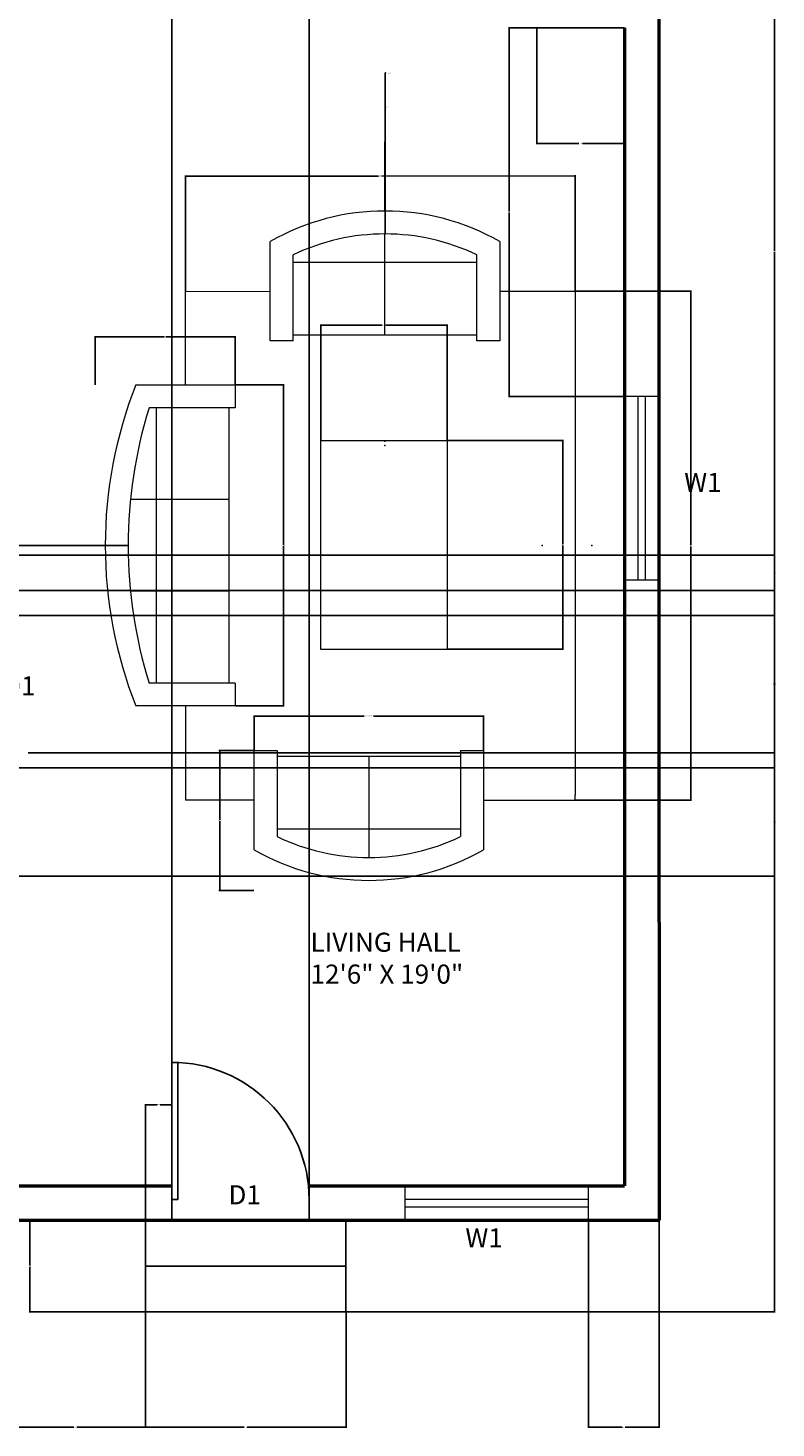
# Model space of a CAD drawing. Units: inches. Extents: x 437 to 811, y 2074 to 2699.
# Tile 2 of 4: x 615 to 811, y 2074 to 2441. Entities that reach past the tile are written whole.
import ezdxf

# ---------------------------------------------------------------- set-up
doc = ezdxf.new("R2010")
doc.units = ezdxf.units.IN
for name, color, linetype, lineweight in [('A-ANNO-DIMS', 2, 'Continuous', 18), ('A-ANNO-TEXT', 7, 'Continuous', 18), ('A-AREA-IDEN', 7, 'Continuous', 25), ('A-DOOR', 4, 'Continuous', 25), ('A-FLOR-STRS', 7, 'Continuous', 25), ('A-FURN', 8, 'Continuous', 18), ('A-GLAZ', 4, 'Continuous', 18), ('A-WALL', 7, 'Continuous', 50)]:
    doc.layers.add(name, color=color, linetype=linetype, lineweight=lineweight)
doc.styles.get("Standard").update_dxf_attribs({"font": 'arial.ttf'})
doc.dimstyles.get("Standard").update_dxf_attribs({"dimtxt": 0.18, "dimasz": 0.18, "dimexe": 0.18, "dimexo": 0.0625, "dimgap": 0.09, "dimtad": 0, "dimtih": 1, "dimtoh": 1, "dimdec": 4, "dimzin": 0, "dimdsep": 46, "dimtxsty": 'Standard', "dimcen": 0.09, "dimadec": 0, "dimazin": 0, "dimtfac": 1, "dimtdec": 4, "dimtofl": 0, "dimtmove": 0, "dimatfit": 3, "dimfxl": 1, "dimtolj": 1, "dimtzin": 0, "dimarcsym": 0})

# ---------------------------------------------------------------- blocks, each defined once
blk = doc.blocks.new('Sofa - Roundback 7 ft.')
for p, q in [((-12.00002, -32.4421), (-12.00003, -6.5971)), ((11.99997, -32.4421), (11.99998, -6.5971)), ((-36.000027, -34), (-36.000027, -11.4696)), ((-35.999844, -13.3819), (35.9998, -13.3819)), ((35.99998, -34), (35.99998, -11.4696)), ((-36.000027, -32.4421), (35.99998, -32.4421))]:
    blk.add_line(p, q)
for points in [[(-36.000027, -34), (-42.000027, -34), (-42.000027, -8)], [(41.99998, -8), (41.99998, -34), (35.99998, -34)]]:
    blk.add_lwpolyline(points)
for centre, radius, start, end in [((0, -114.25), 114.25, 68.43141, 111.5686), ((-0.00001, -127.1968), 121.1968, 72.72033, 107.2797)]:
    blk.add_arc(centre, radius, start, end)
blk = doc.blocks.new('Sofa - Roundback Loveseat 5 ft.')
for p, q in [((0, -32.44198), (0, -5.99998)), ((-24, -33.99998), (-24, -11.46958)), ((-23.9998, -13.38178), (23.99986, -13.38178)), ((24.00004, -33.99998), (24.00004, -11.46958)), ((-24, -32.44198), (24.00004, -32.44198))]:
    blk.add_line(p, q)
for points in [[(-24, -33.99998), (-30, -33.99998), (-30, -7.99998)], [(30.00004, -7.99998), (30.00004, -33.99998), (24.00004, -33.99998)]]:
    blk.add_lwpolyline(points)
for centre, radius, start, end in [((0, -60.24998), 60.24998, 60.13715, 119.8628), ((0, -61.38438), 55.38444, 64.32083, 115.6792)]:
    blk.add_arc(centre, radius, start, end)
blk = doc.blocks.new('*U10')
for p, q in [((0, 0), (0, -6)), ((40, 0), (40, -6))]:
    blk.add_line(p, q)
blk.add_lwpolyline([(0, 0), (0, 40), (1.75, 40), (1.75, 0)], close=True)
blk.add_arc((0, 0), 40, 0, 90)
blk = doc.blocks.new('WIN-W1-48IN')
for p, q in [((0, 5.5), (48, 5.5)), ((0, 3.5), (48, 3.5))]:
    blk.add_line(p, q)
blk.add_lwpolyline([(0, 0), (48, 0), (48, 9), (0, 9)], close=True)
blk = doc.blocks.new('*D26')
at = {"layer": 'A-ANNO-DIMS', "color": 0, "lineweight": -2, "transparency": 16777216}
for p, q in [((674.12, 2251.79), (674.12, 2260.91)), ((674.3, 2260.73), (702.89, 2260.73)), ((733.94, 2260.73), (705.34, 2260.73)), ((734.12, 2251.79), (734.12, 2260.91))]:
    blk.add_line(p, q, dxfattribs=at)
at = {"layer": 'A-ANNO-DIMS', "color": 0, "transparency": 16777216}
for points in [[(674.3, 2260.76), (674.3, 2260.7), (674.12, 2260.73)], [(733.94, 2260.76), (733.94, 2260.7), (734.12, 2260.73)]]:
    blk.add_solid(points, dxfattribs=at)
at = {"layer": 'Defpoints', "color": 0, "transparency": 16777216}
for p in [(674.12, 2260.73), (674.12, 2251.73), (734.12, 2251.73)]:
    blk.add_point(p, dxfattribs=at)
at = {"layer": 'A-ANNO-DIMS', "color": 0, "transparency": 16777216, "insert": (704.12, 2260.73), "char_height": 0.18, "attachment_point": 5}
blk.add_mtext('\\A1;LOVESEAT 60 TYP.', dxfattribs=at)
blk = doc.blocks.new('*D27')
at = {"layer": 'A-ANNO-DIMS', "color": 0, "lineweight": -2, "transparency": 16777216}
for p, q in [((674.05, 2251.73), (664.94, 2251.73)), ((665.12, 2251.55), (665.12, 2233.58)), ((665.12, 2215.25), (665.12, 2233.22)), ((674.05, 2215.07), (664.94, 2215.07))]:
    blk.add_line(p, q, dxfattribs=at)
at = {"layer": 'A-ANNO-DIMS', "color": 0, "transparency": 16777216}
for points in [[(665.09, 2251.55), (665.15, 2251.55), (665.12, 2251.73)], [(665.09, 2215.25), (665.15, 2215.25), (665.12, 2215.07)]]:
    blk.add_solid(points, dxfattribs=at)
at = {"layer": 'Defpoints', "color": 0, "transparency": 16777216}
for p in [(674.12, 2251.73), (665.12, 2215.07), (674.12, 2215.07)]:
    blk.add_point(p, dxfattribs=at)
at = {"layer": 'A-ANNO-DIMS', "color": 0, "transparency": 16777216, "insert": (665.12, 2233.4), "char_height": 0.18, "attachment_point": 5}
blk.add_mtext('\\A1;37 TYP.', dxfattribs=at)
blk = doc.blocks.new('*D36')
at = {"layer": 'A-ANNO-DIMS', "color": 0, "lineweight": -2, "transparency": 16777216}
for p, q in [((669.25, 2347.38), (681.97, 2347.38)), ((681.79, 2347.2), (681.79, 2305.57)), ((681.79, 2263.56), (681.79, 2305.2)), ((669.25, 2263.38), (681.97, 2263.38))]:
    blk.add_line(p, q, dxfattribs=at)
at = {"layer": 'A-ANNO-DIMS', "color": 0, "transparency": 16777216}
for points in [[(681.76, 2347.2), (681.82, 2347.2), (681.79, 2347.38)], [(681.76, 2263.56), (681.82, 2263.56), (681.79, 2263.38)]]:
    blk.add_solid(points, dxfattribs=at)
at = {"layer": 'Defpoints', "color": 0, "transparency": 16777216}
for p in [(669.19, 2347.38), (681.79, 2347.38), (669.19, 2263.38)]:
    blk.add_point(p, dxfattribs=at)
at = {"layer": 'A-ANNO-DIMS', "color": 0, "transparency": 16777216, "insert": (681.79, 2305.38), "char_height": 0.18, "attachment_point": 5}
blk.add_mtext('\\A1;SOFA 84', dxfattribs=at)
blk = doc.blocks.new('*D37')
at = {"layer": 'A-ANNO-DIMS', "color": 0, "lineweight": -2, "transparency": 16777216}
for p, q in [((632.53, 2347.44), (632.53, 2360.16)), ((632.71, 2359.98), (650.64, 2359.98)), ((669.01, 2359.98), (651.08, 2359.98)), ((669.19, 2347.44), (669.19, 2360.16))]:
    blk.add_line(p, q, dxfattribs=at)
at = {"layer": 'A-ANNO-DIMS', "color": 0, "transparency": 16777216}
for points in [[(632.71, 2360.01), (632.71, 2359.95), (632.53, 2359.98)], [(669.01, 2360.01), (669.01, 2359.95), (669.19, 2359.98)]]:
    blk.add_solid(points, dxfattribs=at)
at = {"layer": 'Defpoints', "color": 0, "transparency": 16777216}
for p in [(632.53, 2359.98), (632.53, 2347.38), (669.19, 2347.38)]:
    blk.add_point(p, dxfattribs=at)
at = {"layer": 'A-ANNO-DIMS', "color": 0, "transparency": 16777216, "insert": (650.86, 2359.98), "char_height": 0.18, "attachment_point": 5}
blk.add_mtext('\\A1;37', dxfattribs=at)
blk = doc.blocks.new('*D42')
at = {"layer": 'A-ANNO-DIMS', "color": 0, "lineweight": -2, "transparency": 16777216}
for p, q in [((645.63, 2128.8), (615.31, 2128.8)), ((615.49, 2128.62), (615.49, 2116.98)), ((615.49, 2104.98), (615.49, 2116.62)), ((645.63, 2104.8), (615.31, 2104.8))]:
    blk.add_line(p, q, dxfattribs=at)
at = {"layer": 'A-ANNO-DIMS', "color": 0, "transparency": 16777216}
for points in [[(615.46, 2128.62), (615.52, 2128.62), (615.49, 2128.8)], [(615.46, 2104.98), (615.52, 2104.98), (615.49, 2104.8)]]:
    blk.add_solid(points, dxfattribs=at)
at = {"layer": 'Defpoints', "color": 0, "transparency": 16777216}
for p in [(615.49, 2128.8), (645.69, 2128.8), (645.69, 2104.8)]:
    blk.add_point(p, dxfattribs=at)
at = {"layer": 'A-ANNO-DIMS', "color": 0, "transparency": 16777216, "insert": (615.49, 2116.8), "char_height": 0.18, "attachment_point": 5}
blk.add_mtext('\\A1;24', dxfattribs=at)
blk = doc.blocks.new('*D43')
at = {"layer": 'A-ANNO-DIMS', "color": 0, "lineweight": -2, "transparency": 16777216}
for p, q in [((645.69, 2104.74), (645.69, 2074.42)), ((698.15, 2104.74), (698.15, 2074.42)), ((645.87, 2074.6), (671.53, 2074.6)), ((697.97, 2074.6), (672.31, 2074.6))]:
    blk.add_line(p, q, dxfattribs=at)
at = {"layer": 'A-ANNO-DIMS', "color": 0, "transparency": 16777216}
for points in [[(645.87, 2074.63), (645.87, 2074.57), (645.69, 2074.6)], [(697.97, 2074.63), (697.97, 2074.57), (698.15, 2074.6)]]:
    blk.add_solid(points, dxfattribs=at)
at = {"layer": 'Defpoints', "color": 0, "transparency": 16777216}
for p in [(645.69, 2104.8), (698.15, 2104.8), (698.15, 2074.6)]:
    blk.add_point(p, dxfattribs=at)
at = {"layer": 'A-ANNO-DIMS', "color": 0, "transparency": 16777216, "insert": (671.92, 2074.6), "char_height": 0.18, "attachment_point": 5}
blk.add_mtext('\\A1;52.46', dxfattribs=at)
blk = doc.blocks.new('*D44')
at = {"layer": 'A-ANNO-DIMS', "color": 0, "lineweight": -2, "transparency": 16777216}
for p, q in [((609, 2137.74), (609, 2074.42)), ((645.69, 2104.74), (645.69, 2074.42)), ((609.18, 2074.6), (626.95, 2074.6)), ((645.51, 2074.6), (627.74, 2074.6))]:
    blk.add_line(p, q, dxfattribs=at)
at = {"layer": 'A-ANNO-DIMS', "color": 0, "transparency": 16777216}
for points in [[(609.18, 2074.63), (609.18, 2074.57), (609, 2074.6)], [(645.51, 2074.63), (645.51, 2074.57), (645.69, 2074.6)]]:
    blk.add_solid(points, dxfattribs=at)
at = {"layer": 'Defpoints', "color": 0, "transparency": 16777216}
for p in [(609, 2137.8), (645.69, 2104.8), (645.69, 2074.6)]:
    blk.add_point(p, dxfattribs=at)
at = {"layer": 'A-ANNO-DIMS', "color": 0, "transparency": 16777216, "insert": (627.35, 2074.6), "char_height": 0.18, "attachment_point": 5}
blk.add_mtext('\\A1;36.69', dxfattribs=at)
blk = doc.blocks.new('*D45')
at = {"layer": 'A-ANNO-DIMS', "color": 0, "lineweight": -2, "transparency": 16777216}
for p, q in [((652.6, 2128.86), (652.6, 2690.18)), ((652.78, 2690), (670.09, 2690)), ((688.34, 2690), (671.02, 2690)), ((688.52, 2128.86), (688.52, 2690.18))]:
    blk.add_line(p, q, dxfattribs=at)
at = {"layer": 'A-ANNO-DIMS', "color": 0, "transparency": 16777216}
for points in [[(652.78, 2690.03), (652.78, 2689.97), (652.6, 2690)], [(688.34, 2690.03), (688.34, 2689.97), (688.52, 2690)]]:
    blk.add_solid(points, dxfattribs=at)
at = {"layer": 'Defpoints', "color": 0, "transparency": 16777216}
for p in [(688.52, 2690), (652.6, 2128.8), (688.52, 2128.8)]:
    blk.add_point(p, dxfattribs=at)
at = {"layer": 'A-ANNO-DIMS', "color": 0, "transparency": 16777216, "insert": (670.56, 2690), "char_height": 0.18, "attachment_point": 5}
blk.add_mtext('\\A1;35.924', dxfattribs=at)
blk = doc.blocks.new('*D46')
at = {"layer": 'A-ANNO-DIMS', "color": 0, "lineweight": -2, "transparency": 16777216}
for p, q in [((645.69, 2128.86), (645.69, 2159.18)), ((645.87, 2159), (648.75, 2159)), ((652.42, 2159), (649.54, 2159)), ((652.6, 2128.86), (652.6, 2159.18))]:
    blk.add_line(p, q, dxfattribs=at)
at = {"layer": 'A-ANNO-DIMS', "color": 0, "transparency": 16777216}
for points in [[(645.87, 2159.03), (645.87, 2158.97), (645.69, 2159)], [(652.42, 2159.03), (652.42, 2158.97), (652.6, 2159)]]:
    blk.add_solid(points, dxfattribs=at)
at = {"layer": 'Defpoints', "color": 0, "transparency": 16777216}
for p in [(652.6, 2159), (645.69, 2128.8), (652.6, 2128.8)]:
    blk.add_point(p, dxfattribs=at)
at = {"layer": 'A-ANNO-DIMS', "color": 0, "transparency": 16777216, "insert": (649.14, 2159), "char_height": 0.18, "attachment_point": 5}
blk.add_mtext('\\A1;6.903', dxfattribs=at)
blk = doc.blocks.new('*D47')
at = {"layer": 'A-ANNO-DIMS', "color": 0, "lineweight": -2, "transparency": 16777216}
for p, q in [((761.56, 2128.74), (761.56, 2074.42)), ((780, 2128.74), (780, 2074.42)), ((761.74, 2074.6), (770.4, 2074.6)), ((779.82, 2074.6), (771.17, 2074.6))]:
    blk.add_line(p, q, dxfattribs=at)
at = {"layer": 'A-ANNO-DIMS', "color": 0, "transparency": 16777216}
for points in [[(761.74, 2074.63), (761.74, 2074.57), (761.56, 2074.6)], [(779.82, 2074.63), (779.82, 2074.57), (780, 2074.6)]]:
    blk.add_solid(points, dxfattribs=at)
at = {"layer": 'Defpoints', "color": 0, "transparency": 16777216}
for p in [(761.56, 2128.8), (780, 2128.8), (780, 2074.6)]:
    blk.add_point(p, dxfattribs=at)
at = {"layer": 'A-ANNO-DIMS', "color": 0, "transparency": 16777216, "insert": (770.78, 2074.6), "char_height": 0.18, "attachment_point": 5}
blk.add_mtext('\\A1;18.44', dxfattribs=at)
blk = doc.blocks.new('*D55')
at = {"layer": 'A-ANNO-DIMS', "color": 0, "lineweight": -2, "transparency": 16777216}
for p, q in [((770.94, 2440.8), (740.62, 2440.8)), ((740.8, 2440.62), (740.8, 2392.78)), ((740.8, 2344.57), (740.8, 2392.41)), ((770.94, 2344.39), (740.62, 2344.39))]:
    blk.add_line(p, q, dxfattribs=at)
at = {"layer": 'A-ANNO-DIMS', "color": 0, "transparency": 16777216}
for points in [[(740.77, 2440.62), (740.83, 2440.62), (740.8, 2440.8)], [(740.77, 2344.57), (740.83, 2344.57), (740.8, 2344.39)]]:
    blk.add_solid(points, dxfattribs=at)
at = {"layer": 'Defpoints', "color": 0, "transparency": 16777216}
for p in [(740.8, 2440.8), (771, 2440.8), (771, 2344.39)]:
    blk.add_point(p, dxfattribs=at)
at = {"layer": 'A-ANNO-DIMS', "color": 0, "transparency": 16777216, "insert": (740.8, 2392.59), "char_height": 0.18, "attachment_point": 5}
blk.add_mtext('\\A1;96.4', dxfattribs=at)
blk = doc.blocks.new('*D64')
at = {"layer": 'A-ANNO-DIMS', "color": 0, "lineweight": -2, "transparency": 16777216}
for p, q in [((615.07, 2287.06), (810.38, 2287.06)), ((810.2, 2286.88), (810.2, 2269.28)), ((810.2, 2251.31), (810.2, 2268.91)), ((615.07, 2251.13), (810.38, 2251.13))]:
    blk.add_line(p, q, dxfattribs=at)
at = {"layer": 'A-ANNO-DIMS', "color": 0, "transparency": 16777216}
for points in [[(810.17, 2286.88), (810.23, 2286.88), (810.2, 2287.06)], [(810.17, 2251.31), (810.23, 2251.31), (810.2, 2251.13)]]:
    blk.add_solid(points, dxfattribs=at)
at = {"layer": 'Defpoints', "color": 0, "transparency": 16777216}
for p in [(615, 2287.06), (810.2, 2287.06), (615, 2251.13)]:
    blk.add_point(p, dxfattribs=at)
at = {"layer": 'A-ANNO-DIMS', "color": 0, "transparency": 16777216, "insert": (810.2, 2269.1), "char_height": 0.18, "attachment_point": 5}
blk.add_mtext('\\A1;35.924', dxfattribs=at)
blk = doc.blocks.new('*D65')
at = {"layer": 'A-ANNO-DIMS', "color": 0, "lineweight": -2, "transparency": 16777216}
for p, q in [((609.07, 2302.8), (810.38, 2302.8)), ((810.2, 2302.62), (810.2, 2295.11)), ((810.2, 2287.23), (810.2, 2294.74)), ((609.07, 2287.05), (810.38, 2287.05))]:
    blk.add_line(p, q, dxfattribs=at)
at = {"layer": 'A-ANNO-DIMS', "color": 0, "transparency": 16777216}
for points in [[(810.17, 2302.62), (810.23, 2302.62), (810.2, 2302.8)], [(810.17, 2287.23), (810.23, 2287.23), (810.2, 2287.05)]]:
    blk.add_solid(points, dxfattribs=at)
at = {"layer": 'Defpoints', "color": 0, "transparency": 16777216}
for p in [(609, 2302.8), (810.2, 2302.8), (609, 2287.05)]:
    blk.add_point(p, dxfattribs=at)
at = {"layer": 'A-ANNO-DIMS', "color": 0, "transparency": 16777216, "insert": (810.2, 2294.93), "char_height": 0.18, "attachment_point": 5}
blk.add_mtext('\\A1;15.747', dxfattribs=at)
blk = doc.blocks.new('*D68')
at = {"layer": 'A-ANNO-DIMS', "color": 0, "lineweight": -2, "transparency": 16777216}
for p, q in [((609.07, 2247.18), (810.38, 2247.18)), ((810.2, 2247), (810.2, 2233.17)), ((810.2, 2218.98), (810.2, 2232.81)), ((609.07, 2218.8), (810.38, 2218.8))]:
    blk.add_line(p, q, dxfattribs=at)
at = {"layer": 'A-ANNO-DIMS', "color": 0, "transparency": 16777216}
for points in [[(810.17, 2247), (810.23, 2247), (810.2, 2247.18)], [(810.17, 2218.98), (810.23, 2218.98), (810.2, 2218.8)]]:
    blk.add_solid(points, dxfattribs=at)
at = {"layer": 'Defpoints', "color": 0, "transparency": 16777216}
for p in [(609, 2247.18), (810.2, 2247.18), (609, 2218.8)]:
    blk.add_point(p, dxfattribs=at)
at = {"layer": 'A-ANNO-DIMS', "color": 0, "transparency": 16777216, "insert": (810.2, 2232.99), "char_height": 0.18, "attachment_point": 5}
blk.add_mtext('\\A1;28.384', dxfattribs=at)
blk = doc.blocks.new('*D70')
at = {"layer": 'A-ANNO-DIMS', "color": 0, "lineweight": -2, "transparency": 16777216}
for p, q in [((505.98, 2302.8), (810.38, 2302.8)), ((810.2, 2302.62), (810.2, 2298.36)), ((810.2, 2293.74), (810.2, 2298)), ((500.46, 2293.56), (810.38, 2293.56))]:
    blk.add_line(p, q, dxfattribs=at)
at = {"layer": 'A-ANNO-DIMS', "color": 0, "transparency": 16777216}
for points in [[(810.17, 2302.62), (810.23, 2302.62), (810.2, 2302.8)], [(810.17, 2293.74), (810.23, 2293.74), (810.2, 2293.56)]]:
    blk.add_solid(points, dxfattribs=at)
at = {"layer": 'Defpoints', "color": 0, "transparency": 16777216}
for p in [(505.92, 2302.8), (810.2, 2302.8), (500.4, 2293.56)]:
    blk.add_point(p, dxfattribs=at)
at = {"layer": 'A-ANNO-DIMS', "color": 0, "transparency": 16777216, "insert": (810.2, 2298.18), "char_height": 0.18, "attachment_point": 5}
blk.add_mtext('\\A1;9.244', dxfattribs=at)
blk = doc.blocks.new('*D78')
at = {"layer": 'A-ANNO-DIMS', "color": 0, "lineweight": -2, "transparency": 16777216}
for p, q in [((748.06, 2440.74), (748.06, 2410.42)), ((771, 2440.74), (771, 2410.42)), ((748.24, 2410.6), (759.07, 2410.6)), ((770.82, 2410.6), (760, 2410.6))]:
    blk.add_line(p, q, dxfattribs=at)
at = {"layer": 'A-ANNO-DIMS', "color": 0, "transparency": 16777216}
for points in [[(748.24, 2410.63), (748.24, 2410.57), (748.06, 2410.6)], [(770.82, 2410.63), (770.82, 2410.57), (771, 2410.6)]]:
    blk.add_solid(points, dxfattribs=at)
at = {"layer": 'Defpoints', "color": 0, "transparency": 16777216}
for p in [(748.06, 2440.8), (771, 2440.8), (748.06, 2410.6)]:
    blk.add_point(p, dxfattribs=at)
at = {"layer": 'A-ANNO-DIMS', "color": 0, "transparency": 16777216, "insert": (759.53, 2410.6), "char_height": 0.18, "attachment_point": 5}
blk.add_mtext('\\A1;22.947', dxfattribs=at)
blk = doc.blocks.new('*D82')
at = {"layer": 'A-ANNO-DIMS', "color": 0, "lineweight": -2, "transparency": 16777216}
for p, q in [((691.53, 2332.93), (691.53, 2363.24)), ((724.63, 2332.93), (724.63, 2363.24)), ((691.71, 2363.06), (707.62, 2363.06)), ((724.45, 2363.06), (708.55, 2363.06))]:
    blk.add_line(p, q, dxfattribs=at)
at = {"layer": 'A-ANNO-DIMS', "color": 0, "transparency": 16777216}
for points in [[(691.71, 2363.09), (691.71, 2363.03), (691.53, 2363.06)], [(724.45, 2363.09), (724.45, 2363.03), (724.63, 2363.06)]]:
    blk.add_solid(points, dxfattribs=at)
at = {"layer": 'Defpoints', "color": 0, "transparency": 16777216}
for p in [(724.63, 2363.06), (691.53, 2332.86), (724.63, 2332.86)]:
    blk.add_point(p, dxfattribs=at)
at = {"layer": 'A-ANNO-DIMS', "color": 0, "transparency": 16777216, "insert": (708.08, 2363.06), "char_height": 0.18, "attachment_point": 5}
blk.add_mtext('\\A1;33.096', dxfattribs=at)
blk = doc.blocks.new('*D83')
at = {"layer": 'A-ANNO-DIMS', "color": 0, "lineweight": -2, "transparency": 16777216}
for p, q in [((724.69, 2332.86), (755.01, 2332.86)), ((754.83, 2332.68), (754.83, 2305.71)), ((754.83, 2278.38), (754.83, 2305.35)), ((724.69, 2278.2), (755.01, 2278.2))]:
    blk.add_line(p, q, dxfattribs=at)
at = {"layer": 'A-ANNO-DIMS', "color": 0, "transparency": 16777216}
for points in [[(754.8, 2332.68), (754.86, 2332.68), (754.83, 2332.86)], [(754.8, 2278.38), (754.86, 2278.38), (754.83, 2278.2)]]:
    blk.add_solid(points, dxfattribs=at)
at = {"layer": 'Defpoints', "color": 0, "transparency": 16777216}
for p in [(724.63, 2332.86), (724.63, 2278.2), (754.83, 2278.2)]:
    blk.add_point(p, dxfattribs=at)
at = {"layer": 'A-ANNO-DIMS', "color": 0, "transparency": 16777216, "insert": (754.83, 2305.53), "char_height": 0.18, "attachment_point": 5}
blk.add_mtext('\\A1;54.67', dxfattribs=at)
blk = doc.blocks.new('*D84')
at = {"layer": 'A-ANNO-DIMS', "color": 0, "lineweight": -2, "transparency": 16777216}
for p, q in [((656.19, 2371.88), (656.17, 2402.2)), ((656.35, 2402.02), (706.68, 2402.06)), ((757.9, 2402.1), (707.56, 2402.06)), ((758.1, 2371.97), (758.08, 2402.28))]:
    blk.add_line(p, q, dxfattribs=at)
at = {"layer": 'A-ANNO-DIMS', "color": 0, "transparency": 16777216}
for points in [[(656.35, 2402.05), (656.35, 2401.99), (656.17, 2402.02)], [(757.9, 2402.13), (757.9, 2402.07), (758.08, 2402.1)]]:
    blk.add_solid(points, dxfattribs=at)
at = {"layer": 'Defpoints', "color": 0, "transparency": 16777216}
for p in [(758.08, 2402.1), (656.19, 2371.82), (758.1, 2371.9)]:
    blk.add_point(p, dxfattribs=at)
at = {"layer": 'A-ANNO-DIMS', "color": 0, "transparency": 16777216, "insert": (707.12, 2402.06), "char_height": 0.18, "attachment_point": 5}
blk.add_mtext('\\A1;101.91', dxfattribs=at)
blk = doc.blocks.new('*D85')
at = {"layer": 'A-ANNO-DIMS', "color": 0, "lineweight": -2, "transparency": 16777216}
for p, q in [((758.17, 2371.9), (788.48, 2371.9)), ((788.3, 2371.72), (788.3, 2305.5)), ((788.3, 2238.91), (788.3, 2305.14)), ((758.17, 2238.73), (788.48, 2238.73))]:
    blk.add_line(p, q, dxfattribs=at)
at = {"layer": 'A-ANNO-DIMS', "color": 0, "transparency": 16777216}
for points in [[(788.27, 2371.72), (788.33, 2371.72), (788.3, 2371.9)], [(788.27, 2238.91), (788.33, 2238.91), (788.3, 2238.73)]]:
    blk.add_solid(points, dxfattribs=at)
at = {"layer": 'Defpoints', "color": 0, "transparency": 16777216}
for p in [(758.1, 2371.9), (758.1, 2238.73), (788.3, 2238.73)]:
    blk.add_point(p, dxfattribs=at)
at = {"layer": 'A-ANNO-DIMS', "color": 0, "transparency": 16777216, "insert": (788.3, 2305.32), "char_height": 0.18, "attachment_point": 5}
blk.add_mtext('\\A1;133.17', dxfattribs=at)
blk = doc.blocks.new('*D87')
at = {"layer": 'A-ANNO-DIMS', "color": 0, "lineweight": -2, "transparency": 16777216}
for p, q in [((780.07, 2659.8), (810.38, 2659.8)), ((810.2, 2659.62), (810.2, 2382.48)), ((810.2, 2104.98), (810.2, 2382.12)), ((698.21, 2104.8), (810.38, 2104.8))]:
    blk.add_line(p, q, dxfattribs=at)
at = {"layer": 'A-ANNO-DIMS', "color": 0, "transparency": 16777216}
for points in [[(810.17, 2659.62), (810.23, 2659.62), (810.2, 2659.8)], [(810.17, 2104.98), (810.23, 2104.98), (810.2, 2104.8)]]:
    blk.add_solid(points, dxfattribs=at)
at = {"layer": 'Defpoints', "color": 0, "transparency": 16777216}
for p in [(780, 2659.8), (810.2, 2659.8), (698.15, 2104.8)]:
    blk.add_point(p, dxfattribs=at)
at = {"layer": 'A-ANNO-DIMS', "color": 0, "transparency": 16777216, "insert": (810.2, 2382.3), "char_height": 0.18, "attachment_point": 5}
blk.add_mtext('\\A1;555', dxfattribs=at)
blk = doc.blocks.new('*D88')
at = {"layer": 'A-ANNO-DIMS', "color": 0, "lineweight": -2, "transparency": 16777216}
for p, q in [((568.95, 2305.38), (641.01, 2305.38)), ((762.3, 2305.38), (762.48, 2305.38)), ((762.39, 2305.29), (762.39, 2305.47))]:
    blk.add_line(p, q, dxfattribs=at)
at = {"layer": 'A-ANNO-DIMS', "color": 0, "transparency": 16777216}
blk.add_solid([(641.01, 2305.41), (641.01, 2305.35), (641.19, 2305.38)], dxfattribs=at)
at = {"layer": 'Defpoints', "color": 0, "transparency": 16777216}
for p in [(641.19, 2305.38), (762.39, 2305.38)]:
    blk.add_point(p, dxfattribs=at)
at = {"layer": 'A-ANNO-DIMS', "color": 0, "transparency": 16777216, "insert": (568.47, 2305.38), "char_height": 0.18, "attachment_point": 5}
blk.add_mtext('\\A1;R121.2', dxfattribs=at)
blk = doc.blocks.new('*D89')
at = {"layer": 'A-ANNO-DIMS', "color": 0, "lineweight": -2, "transparency": 16777216}
for p, q in [((566.64, 2305.38), (635.01, 2305.38)), ((749.35, 2305.38), (749.53, 2305.38)), ((749.44, 2305.29), (749.44, 2305.47))]:
    blk.add_line(p, q, dxfattribs=at)
at = {"layer": 'A-ANNO-DIMS', "color": 0, "transparency": 16777216}
blk.add_solid([(635.01, 2305.41), (635.01, 2305.35), (635.19, 2305.38)], dxfattribs=at)
at = {"layer": 'Defpoints', "color": 0, "transparency": 16777216}
for p in [(635.19, 2305.38), (749.44, 2305.38)]:
    blk.add_point(p, dxfattribs=at)
at = {"layer": 'A-ANNO-DIMS', "color": 0, "transparency": 16777216, "insert": (566.09, 2305.38), "char_height": 0.18, "attachment_point": 5}
blk.add_mtext('\\A1;R114.25', dxfattribs=at)
blk = doc.blocks.new('*D90')
at = {"layer": 'A-ANNO-DIMS', "color": 0, "lineweight": -2, "transparency": 16777216}
for p, q in [((708.53, 2429.05), (708.35, 2429.05)), ((708.35, 2429.05), (708.34, 2393.08)), ((708.25, 2332.65), (708.43, 2332.65)), ((708.34, 2332.56), (708.34, 2332.74))]:
    blk.add_line(p, q, dxfattribs=at)
at = {"layer": 'A-ANNO-DIMS', "color": 0, "transparency": 16777216}
blk.add_solid([(708.32, 2393.08), (708.38, 2393.08), (708.34, 2392.9)], dxfattribs=at)
at = {"layer": 'Defpoints', "color": 0, "transparency": 16777216}
for p in [(708.34, 2392.9), (708.34, 2332.65)]:
    blk.add_point(p, dxfattribs=at)
at = {"layer": 'A-ANNO-DIMS', "color": 0, "transparency": 16777216, "insert": (709.2, 2429.05), "char_height": 0.18, "attachment_point": 5}
blk.add_mtext('\\A1;2X R60.25', dxfattribs=at)
blk = doc.blocks.new('*D91')
at = {"layer": 'A-ANNO-DIMS', "color": 0, "lineweight": -2, "transparency": 16777216}
for p, q in [((708.53, 2420.14), (708.35, 2420.14)), ((708.35, 2420.14), (708.35, 2387.08)), ((708.25, 2331.52), (708.43, 2331.52)), ((708.34, 2331.43), (708.34, 2331.61))]:
    blk.add_line(p, q, dxfattribs=at)
at = {"layer": 'A-ANNO-DIMS', "color": 0, "transparency": 16777216}
blk.add_solid([(708.32, 2387.08), (708.38, 2387.08), (708.35, 2386.9)], dxfattribs=at)
at = {"layer": 'Defpoints', "color": 0, "transparency": 16777216}
for p in [(708.35, 2386.9), (708.34, 2331.52)]:
    blk.add_point(p, dxfattribs=at)
at = {"layer": 'A-ANNO-DIMS', "color": 0, "transparency": 16777216, "insert": (709.2, 2420.14), "char_height": 0.18, "attachment_point": 5}
blk.add_mtext('\\A1;2X R55.38', dxfattribs=at)

msp = doc.modelspace()

# ---------------------------------------------------------------- linework, layer by layer
at = {"layer": 'A-FLOR-STRS'}
for p, q in [((645.6926, 2128.7995), (645.6926, 2104.7995)), ((698.148, 2104.7995), (698.148, 2128.7995)), ((698.148, 2116.7995), (645.6926, 2116.7995)), ((645.6926, 2104.7995), (698.148, 2104.7995))]:
    msp.add_line(p, q, dxfattribs=at)
at = {"layer": 'A-FURN'}
for p, q in [((656.1918, 2371.8165), (678.3446, 2371.9048)), ((656.1918, 2347.3821), (656.1918, 2371.8165)), ((738.3446, 2371.9048), (758.1032, 2371.9048)), ((758.1032, 2371.9048), (758.1032, 2240.0335)), ((691.5345, 2332.8641), (724.6301, 2332.8641)), ((691.5345, 2278.1957), (691.5345, 2332.8641)), ((724.6301, 2332.8641), (724.6301, 2278.1957)), ((724.6301, 2278.1957), (691.5345, 2278.1957)), ((656.1918, 2263.3821), (656.1918, 2238.732)), ((674.1158, 2238.732), (656.1918, 2238.732)), ((734.1158, 2238.732), (758.1032, 2238.732)), ((758.1032, 2238.732), (758.1032, 2240.0335))]:
    msp.add_line(p, q, dxfattribs=at)
at = {"layer": 'A-WALL'}
for p, q in [((780.0049, 2206.7995), (780.0049, 2659.7995)), ((771.0049, 2440.7995), (771.0049, 2206.7995)), ((771.0049, 2206.7995), (771.0049, 2137.7995)), ((780.0049, 2206.7995), (780.0049, 2128.7995)), ((477.0049, 2137.7995), (652.5955, 2137.7995)), ((688.3376, 2137.7995), (771.0049, 2137.7995)), ((468.0049, 2128.7995), (658.0738, 2128.7995)), ((658.0738, 2128.7995), (780.0049, 2128.7995))]:
    msp.add_line(p, q, dxfattribs=at)

# ---------------------------------------------------------------- block references
at = {"layer": 'A-DOOR', "xscale": 0.8981017077080947, "yscale": 0.8981017077080947, "zscale": 0.8981017077080947}
msp.add_blockref('*U10', (652.5955, 2134.1881), dxfattribs=at)
at = {"layer": 'A-FURN'}
msp.add_blockref('Sofa - Roundback Loveseat 5 ft.', (708.3446, 2392.9048), dxfattribs=at)
for name, p, rotation in [('Sofa - Roundback 7 ft.', (635.1918, 2305.3821), 90), ('Sofa - Roundback Loveseat 5 ft.', (704.1158, 2217.732), 180)]:
    msp.add_blockref(name, p, dxfattribs=dict(at, rotation=rotation))
at = {"layer": 'A-GLAZ', "rotation": 89.99999999999935}
msp.add_blockref('WIN-W1-48IN', (780.0053, 2296.3904), dxfattribs=at)
at = {"layer": 'A-GLAZ'}
msp.add_blockref('WIN-W1-48IN', (713.5648, 2128.799), dxfattribs=at)

# ---------------------------------------------------------------- texts
at = {"layer": 'A-ANNO-TEXT', "char_height": 5, "width": 52.048983, "attachment_point": 1}
for s, insert in [('W1', (786.5859, 2324.3865)), ('D1', (608.4809, 2271.1388)), ('D1', (667.418, 2137.9547)), ('W1', (729.3635, 2126.6661))]:
    msp.add_mtext(s, dxfattribs=dict(at, insert=insert))
at = {"layer": 'A-AREA-IDEN', "insert": (688.8721, 2204.039), "char_height": 5, "width": 52.048983, "attachment_point": 1}
msp.add_mtext('LIVING HALL\\P12\'6" X 19\'0"', dxfattribs=at)

# ---------------------------------------------------------------- dimensions: what is measured, and where the dimension line sits
at = {"layer": 'A-ANNO-DIMS'}
for base, p1, p2, override, picture, middle in [((688.5196, 2689.9995), (652.5955, 2128.7995), (688.5196, 2128.7995), {"dimdec": 3, "dimlfac": 1, "dimrnd": 0, "dimzin": 0, "dimdsep": 46, "dimlunit": 2}, '*D45', (670.5576, 2689.9995)), ((724.6301, 2363.0641), (691.5345, 2332.8641), (724.6301, 2332.8641), {"dimdec": 3, "dimlfac": 1, "dimrnd": 0, "dimzin": 0, "dimdsep": 46, "dimlunit": 2}, '*D82', (708.0823, 2363.0641)), ((645.6926, 2074.5995), (609.0049, 2137.7995), (645.6926, 2104.7995), {"dimdec": 2, "dimlfac": 1, "dimrnd": 0, "dimzin": 0, "dimdsep": 46, "dimlunit": 2}, '*D44', (627.3487, 2074.5995)), ((780.0049, 2074.5995), (761.5645, 2128.7995), (780.0049, 2128.7995), {"dimdec": 2, "dimlfac": 1, "dimrnd": 0, "dimzin": 0, "dimdsep": 46, "dimlunit": 2}, '*D47', (770.7847, 2074.5995)), ((698.148, 2074.5995), (645.6926, 2104.7995), (698.148, 2104.7995), {"dimdec": 2, "dimlfac": 1, "dimrnd": 0, "dimzin": 0, "dimdsep": 46, "dimlunit": 2}, '*D43', (671.9203, 2074.5995))]:
    dim = msp.add_linear_dim(base=base, p1=p1, p2=p2, dimstyle='Standard', override=override, dxfattribs=at)
    dim.commit()
    dim.dimension.update_dxf_attribs({"geometry": picture, "text_midpoint": middle})
for base, p1, p2, angle, override, picture, middle in [((810.2049, 2659.7995), (698.148, 2104.7995), (780.0049, 2659.7995), 90, {"dimdec": 0, "dimlfac": 1, "dimrnd": 0, "dimzin": 0, "dimdsep": 46, "dimlunit": 2}, '*D87', (810.2049, 2382.2995)), ((740.8049, 2440.7995), (771.0049, 2344.3901), (771.0049, 2440.7995), 90, {"dimdec": 1, "dimlfac": 1, "dimrnd": 0, "dimzin": 0, "dimdsep": 46, "dimlunit": 2}, '*D55', (740.8049, 2392.5948)), ((748.05835, 2410.59945), (771.00488, 2440.79945), (748.05835, 2440.79945), 180, {"dimdec": 3, "dimlfac": 1, "dimrnd": 0, "dimzin": 0, "dimdsep": 46, "dimlunit": 2}, '*D78', (759.53162, 2410.59945)), ((758.077, 2402.1048), (656.1918, 2371.8165), (758.1032, 2371.9048), 0.049627, {"dimdec": 2, "dimlfac": 1, "dimrnd": 0, "dimzin": 0, "dimdsep": 46, "dimlunit": 2}, '*D84', (707.1213, 2402.0607)), ((788.3032, 2238.732), (758.1032, 2371.9048), (758.1032, 2238.732), 270, {"dimdec": 2, "dimlfac": 1, "dimrnd": 0, "dimzin": 0, "dimdsep": 46, "dimlunit": 2}, '*D85', (788.3032, 2305.3184)), ((632.5251, 2359.9821), (669.1918, 2347.3821), (632.5251, 2347.3821), 180, {"dimdec": 0, "dimlfac": 1, "dimrnd": 0, "dimzin": 0, "dimdsep": 46, "dimlunit": 2}, '*D37', (650.8585, 2359.9821)), ((754.8301, 2278.1957), (724.6301, 2332.8641), (724.6301, 2278.1957), 270, {"dimdec": 2, "dimlfac": 1, "dimrnd": 0, "dimzin": 0, "dimdsep": 46, "dimlunit": 2}, '*D83', (754.8301, 2305.5299)), ((810.2049, 2302.7995), (500.4016, 2293.5551), (505.9211, 2302.7995), 90, {"dimdec": 3, "dimlfac": 1, "dimrnd": 0, "dimzin": 0, "dimdsep": 46, "dimlunit": 2}, '*D70', (810.2049, 2298.1773)), ((810.2049, 2302.7995), (609.0049, 2287.0521), (609.0049, 2302.7995), 90, {"dimdec": 3, "dimlfac": 1, "dimrnd": 0, "dimzin": 0, "dimdsep": 46, "dimlunit": 2}, '*D65', (810.2049, 2294.9258)), ((810.2049, 2287.0573), (615.0049, 2251.1333), (615.0049, 2287.0573), 90, {"dimdec": 3, "dimlfac": 1, "dimrnd": 0, "dimzin": 0, "dimdsep": 46, "dimlunit": 2}, '*D64', (810.2049, 2269.0953)), ((810.2049, 2247.1838), (609.0049, 2218.7995), (609.0049, 2247.1838), 90, {"dimdec": 3, "dimlfac": 1, "dimrnd": 0, "dimzin": 0, "dimdsep": 46, "dimlunit": 2}, '*D68', (810.2049, 2232.9916)), ((652.5955, 2158.9995), (645.6926, 2128.7995), (652.5955, 2128.7995), 0, {"dimdec": 3, "dimlfac": 1, "dimrnd": 0, "dimzin": 0, "dimdsep": 46, "dimlunit": 2}, '*D46', (649.1441, 2158.9995)), ((615.4926, 2128.7995), (645.6926, 2104.7995), (645.6926, 2128.7995), 90, {"dimdec": 0, "dimlfac": 1, "dimrnd": 0, "dimzin": 0, "dimdsep": 46, "dimlunit": 2}, '*D42', (615.4926, 2116.7995))]:
    dim = msp.add_linear_dim(base=base, p1=p1, p2=p2, angle=angle, dimstyle='Standard', override=override, dxfattribs=at)
    dim.commit()
    dim.dimension.update_dxf_attribs({"geometry": picture, "text_midpoint": middle})
for center, mpoint, picture, middle in [((708.3446, 2332.6548), (708.345, 2392.9048), '*D90', (709.2007, 2429.0548)), ((708.3446, 2331.5204), (708.345, 2386.9048), '*D91', (709.2002, 2420.1355))]:
    dim = msp.add_radius_dim(center=center, mpoint=mpoint, text='2X <>', dimstyle='Standard', override={"dimdec": 2, "dimlfac": 1, "dimrnd": 0, "dimzin": 0, "dimdsep": 46, "dimlunit": 2}, dxfattribs=at)
    dim.commit()
    dim.dimension.update_dxf_attribs({"geometry": picture, "text_midpoint": middle, "dimtype": 164})
for base, p1, p2, angle, text, picture, middle in [((681.7918, 2347.3821), (669.1918, 2263.3821), (669.1918, 2347.3821), 90, 'SOFA <>', '*D36', (681.7918, 2305.3821)), ((674.1158, 2260.732), (734.1158, 2251.732), (674.1158, 2251.732), 180, 'LOVESEAT <> TYP.', '*D26', (704.1158, 2260.732)), ((665.1158, 2215.0653), (674.1158, 2251.732), (674.1158, 2215.0653), 270, '<> TYP.', '*D27', (665.1158, 2233.3987))]:
    dim = msp.add_linear_dim(base=base, p1=p1, p2=p2, angle=angle, text=text, dimstyle='Standard', override={"dimdec": 0, "dimlfac": 1, "dimrnd": 0, "dimzin": 0, "dimdsep": 46, "dimlunit": 2}, dxfattribs=at)
    dim.commit()
    dim.dimension.update_dxf_attribs({"geometry": picture, "text_midpoint": middle})
for center, mpoint, override, picture, middle in [((749.4418, 2305.3821), (635.1918, 2305.382), {"dimdec": 2, "dimlfac": 1, "dimrnd": 0, "dimzin": 0, "dimdsep": 46, "dimlunit": 2}, '*D89', (566.6418, 2305.3819)), ((762.3886, 2305.3821), (641.1918, 2305.382), {"dimdec": 1, "dimlfac": 1, "dimrnd": 0, "dimzin": 0, "dimdsep": 46, "dimlunit": 2}, '*D88', (568.4737, 2305.382))]:
    dim = msp.add_radius_dim(center=center, mpoint=mpoint, dimstyle='Standard', override=override, dxfattribs=at)
    dim.commit()
    dim.dimension.update_dxf_attribs({"geometry": picture, "text_midpoint": middle, "dimtype": 164})

doc.saveas('drawing.dxf')
